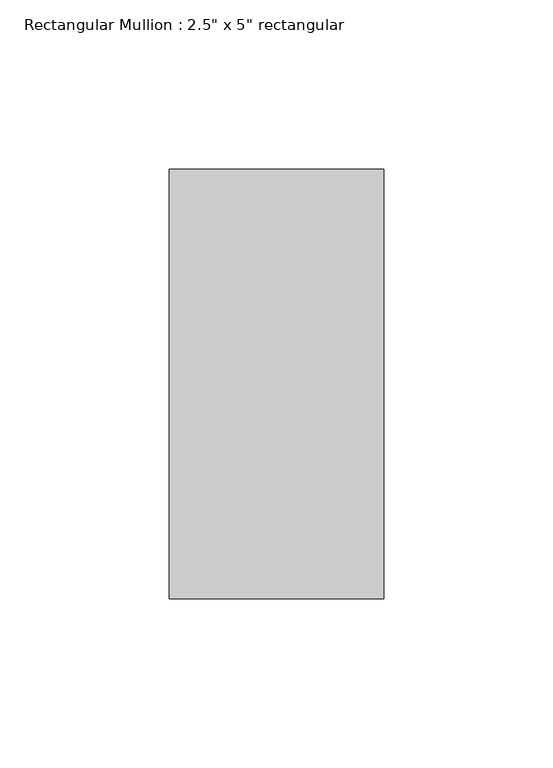
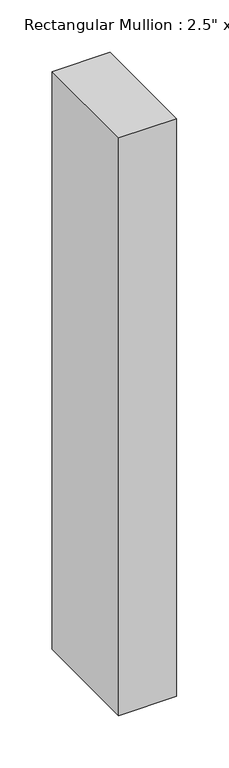
"""IFC4 building model written with IfcOpenShell, lengths in millimetres: member geometry."""

from ifc_helpers import new_model, si_unit, frame, origin, place, context, project, spatial, polyline, outline, extrude, source, transform, mapped, element, save


def member_051277f3(model_context):
    return source(origin(), model_context, "Body", "SweptSolid", [
        extrude(outline(polyline([(0.0, 63.5), (0.0, -63.5), (-63.5, -63.5), (-63.5, 63.5), (0.0, 63.5)])), frame((0.0, 0.0, -673.1), z_axis=(0.0, 0.0, 1.0), x_axis=(1.0, 0.0, 0.0)), (0.0, 0.0, 1.0), 673.1),
    ])


if __name__ == "__main__":
    model = new_model("IFC4")
    model_context = context("Model", 3, world=origin())
    ifc_project = project(units=[si_unit("LENGTHUNIT", "METRE", prefix="MILLI")], contexts=[model_context])
    site = spatial("IfcSite", under=ifc_project)
    building = spatial("IfcBuilding", under=site)
    placement = place(None, origin())
    member_shape = member_051277f3(model_context)
    element("IfcMember", 1, ObjectType="Rectangular Mullion : 2.5\" x 5\" rectangular", at=placement, inside=building, context=model_context, shape_type="MappedRepresentation", body=[
        mapped(member_shape, transform((0.0, 0.0, 0.0), x_axis=(1.0, 0.0, 0.0), y_axis=(0.0, 1.0, 0.0), z_axis=(0.0, 0.0, 1.0))),
    ])
    save(model, "model.ifc")

# Revit data of these elements
# Type "Rectangular Mullion : 2.5\" x 5\" rectangular"
#   built-in parameter 1007304 = 0.416667 (stored number, unit not read)
#   built-in parameter 1007301 = 0.104167 (stored number, unit not read)
#   built-in parameter 1007300 = 0.104167 (stored number, unit not read)
# Element 1 (IfcMember, "Rectangular Mullion : 2.5\" x 5\" rectangular")
#   Materials on its faces: "Aluminum"
# Materials
#   "Aluminum": class "Metal", colour RGB 247 247 247, transparency 0, Description = "Aluminum 6061", Cost = 0
